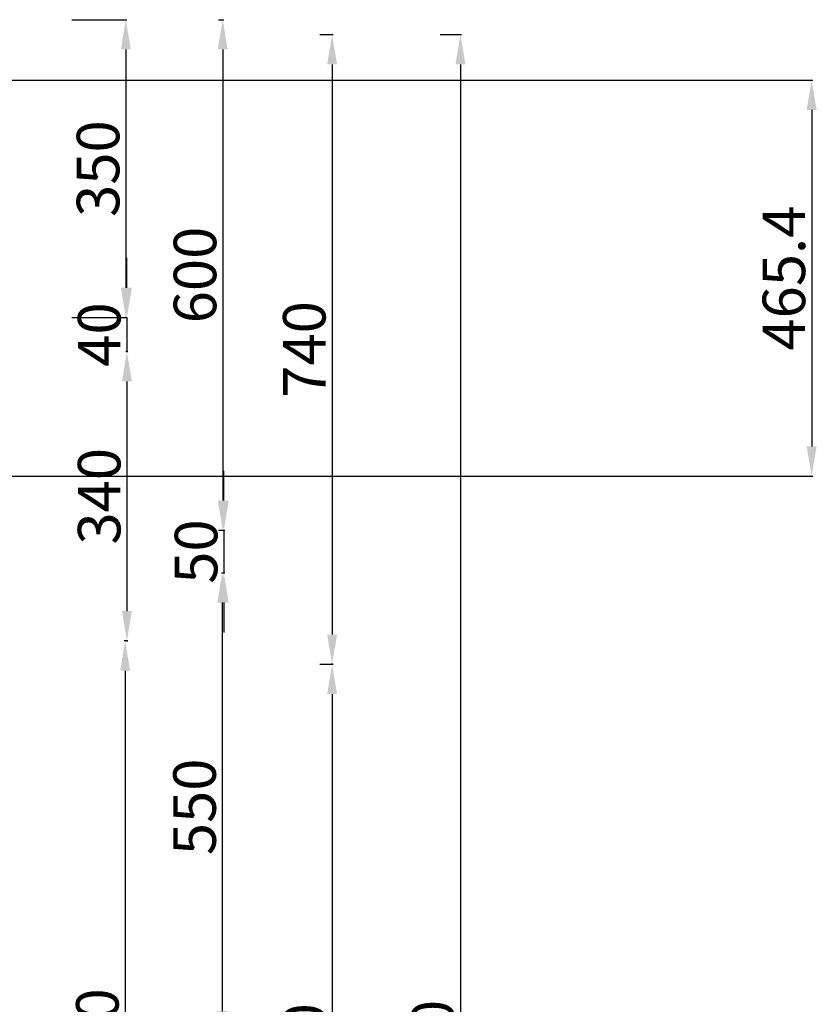
# Model space of a CAD drawing. Units: millimetres. Extents: x 407065 to 421840, y 1168257 to 1177792.
# Tile 10 of 17: x 411029 to 411967, y 1175981 to 1177138. Entities that reach past the tile are written whole.
import ezdxf

# ---------------------------------------------------------------- set-up
doc = ezdxf.new("R2010")
doc.units = ezdxf.units.MM
doc.layers.add('A-ANNO-DIMS', color=6, linetype='Continuous', lineweight=18)
doc.styles.get("Standard").update_dxf_attribs({"font": 'arial.ttf'})
doc.dimstyles.new('ISO-25', dxfattribs={"dimtxt": 50, "dimasz": 35, "dimexe": 1.25, "dimexo": 0.625, "dimtad": 1, "dimdec": 1, "dimtxsty": 'Standard', "dimcen": 35, "dimadec": 0, "dimazin": 0, "dimtfac": 1, "dimtdec": 1, "dimtmove": 0, "dimatfit": 3, "dimfxl": 1, "dimarcsym": 0})

# ---------------------------------------------------------------- blocks, each defined once
blk = doc.blocks.new('*D18')
at = {"layer": 'A-ANNO-DIMS', "color": 0, "lineweight": -2, "transparency": 16777216}
for p, q in [((411090.8, 1177137.8), (411155.4, 1177137.8)), ((411154.2, 1177102.8), (411154.2, 1176822.8)), ((411090.8, 1176787.8), (411155.4, 1176787.8))]:
    blk.add_line(p, q, dxfattribs=at)
at = {"layer": 'A-ANNO-DIMS', "color": 0, "transparency": 16777216}
for points in [[(411148.3, 1177102.8), (411160, 1177102.8), (411154.2, 1177137.8)], [(411148.3, 1176822.8), (411160, 1176822.8), (411154.2, 1176787.8)]]:
    blk.add_solid(points, dxfattribs=at)
at = {"layer": 'Defpoints', "color": 0, "transparency": 16777216}
for p in [(411090.2, 1177137.8), (411090.2, 1176787.8), (411154.2, 1176787.8)]:
    blk.add_point(p, dxfattribs=at)
at = {"layer": 'A-ANNO-DIMS', "color": 0, "transparency": 16777216, "insert": (411128, 1176962.8), "char_height": 50, "attachment_point": 5, "rotation": 90}
blk.add_mtext('350', dxfattribs=at)
blk = doc.blocks.new('*D19')
at = {"layer": 'A-ANNO-DIMS', "color": 0, "lineweight": -2, "transparency": 16777216}
for p, q in [((411155.4, 1176822.8), (411155.4, 1176857.8)), ((411154.8, 1176787.8), (411154.2, 1176787.8)), ((411155.4, 1176787.8), (411155.4, 1176747.8)), ((411154.8, 1176747.8), (411154.2, 1176747.8)), ((411155.4, 1176712.8), (411155.4, 1176677.8))]:
    blk.add_line(p, q, dxfattribs=at)
at = {"layer": 'A-ANNO-DIMS', "color": 0, "transparency": 16777216}
for points in [[(411149.6, 1176822.8), (411161.3, 1176822.8), (411155.4, 1176787.8)], [(411149.6, 1176712.8), (411161.3, 1176712.8), (411155.4, 1176747.8)]]:
    blk.add_solid(points, dxfattribs=at)
at = {"layer": 'Defpoints', "color": 0, "transparency": 16777216}
for p in [(411155.4, 1176787.8), (411155.4, 1176747.8), (411155.4, 1176747.8)]:
    blk.add_point(p, dxfattribs=at)
at = {"layer": 'A-ANNO-DIMS', "color": 0, "transparency": 16777216, "insert": (411129.3, 1176767.8), "char_height": 50, "attachment_point": 5, "rotation": 90}
blk.add_mtext('40', dxfattribs=at)
blk = doc.blocks.new('*D20')
at = {"layer": 'A-ANNO-DIMS', "color": 0, "lineweight": -2, "transparency": 16777216}
for p, q in [((411154.8, 1176747.8), (411156.7, 1176747.8)), ((411155.4, 1176712.8), (411155.4, 1176442.8)), ((411154.8, 1176407.8), (411156.7, 1176407.8))]:
    blk.add_line(p, q, dxfattribs=at)
at = {"layer": 'A-ANNO-DIMS', "color": 0, "transparency": 16777216}
for points in [[(411149.6, 1176712.8), (411161.3, 1176712.8), (411155.4, 1176747.8)], [(411149.6, 1176442.8), (411161.3, 1176442.8), (411155.4, 1176407.8)]]:
    blk.add_solid(points, dxfattribs=at)
at = {"layer": 'Defpoints', "color": 0, "transparency": 16777216}
for p in [(411154.2, 1176747.8), (411154.2, 1176407.8), (411155.4, 1176407.8)]:
    blk.add_point(p, dxfattribs=at)
at = {"layer": 'A-ANNO-DIMS', "color": 0, "transparency": 16777216, "insert": (411129.3, 1176577.8), "char_height": 50, "attachment_point": 5, "rotation": 90}
blk.add_mtext('340', dxfattribs=at)
blk = doc.blocks.new('*D21')
at = {"layer": 'A-ANNO-DIMS', "color": 0, "lineweight": -2, "transparency": 16777216}
for p, q in [((411156.1, 1176407.8), (411152.2, 1176407.8)), ((411153.4, 1176372.8), (411153.4, 1175512.8)), ((411156.1, 1175477.8), (411152.2, 1175477.8))]:
    blk.add_line(p, q, dxfattribs=at)
at = {"layer": 'A-ANNO-DIMS', "color": 0, "transparency": 16777216}
for points in [[(411147.6, 1176372.8), (411159.2, 1176372.8), (411153.4, 1176407.8)], [(411147.6, 1175512.8), (411159.2, 1175512.8), (411153.4, 1175477.8)]]:
    blk.add_solid(points, dxfattribs=at)
at = {"layer": 'Defpoints', "color": 0, "transparency": 16777216}
for p in [(411156.7, 1176407.8), (411153.4, 1175477.8), (411156.7, 1175477.8)]:
    blk.add_point(p, dxfattribs=at)
at = {"layer": 'A-ANNO-DIMS', "color": 0, "transparency": 16777216, "insert": (411127.2, 1175942.8), "char_height": 50, "attachment_point": 5, "rotation": 90}
blk.add_mtext('930', dxfattribs=at)
blk = doc.blocks.new('*D26')
at = {"layer": 'A-ANNO-DIMS', "color": 0, "lineweight": -2, "transparency": 16777216}
for p, q in [((411263.1, 1177137.8), (411269.3, 1177137.8)), ((411268.1, 1177102.8), (411268.1, 1176572.8)), ((411263.1, 1176537.8), (411269.3, 1176537.8))]:
    blk.add_line(p, q, dxfattribs=at)
at = {"layer": 'A-ANNO-DIMS', "color": 0, "transparency": 16777216}
for points in [[(411262.2, 1177102.8), (411273.9, 1177102.8), (411268.1, 1177137.8)], [(411262.2, 1176572.8), (411273.9, 1176572.8), (411268.1, 1176537.8)]]:
    blk.add_solid(points, dxfattribs=at)
at = {"layer": 'Defpoints', "color": 0, "transparency": 16777216}
for p in [(411262.5, 1177137.8), (411262.5, 1176537.8), (411268.1, 1176537.8)]:
    blk.add_point(p, dxfattribs=at)
at = {"layer": 'A-ANNO-DIMS', "color": 0, "transparency": 16777216, "insert": (411241.9, 1176837.8), "char_height": 50, "attachment_point": 5, "rotation": 90}
blk.add_mtext('600', dxfattribs=at)
blk = doc.blocks.new('*D27')
at = {"layer": 'A-ANNO-DIMS', "color": 0, "lineweight": -2, "transparency": 16777216}
for p, q in [((411269.3, 1176572.8), (411269.3, 1176607.8)), ((411266.8, 1176537.8), (411270.6, 1176537.8)), ((411269.3, 1176537.8), (411269.3, 1176487.8)), ((411266.8, 1176487.8), (411270.6, 1176487.8)), ((411269.3, 1176452.8), (411269.3, 1176417.8))]:
    blk.add_line(p, q, dxfattribs=at)
at = {"layer": 'A-ANNO-DIMS', "color": 0, "transparency": 16777216}
for points in [[(411263.5, 1176572.8), (411275.1, 1176572.8), (411269.3, 1176537.8)], [(411263.5, 1176452.8), (411275.1, 1176452.8), (411269.3, 1176487.8)]]:
    blk.add_solid(points, dxfattribs=at)
at = {"layer": 'Defpoints', "color": 0, "transparency": 16777216}
for p in [(411266.2, 1176537.8), (411266.2, 1176487.8), (411269.3, 1176487.8)]:
    blk.add_point(p, dxfattribs=at)
at = {"layer": 'A-ANNO-DIMS', "color": 0, "transparency": 16777216, "insert": (411243.2, 1176512.8), "char_height": 50, "attachment_point": 5, "rotation": 90}
blk.add_mtext('50', dxfattribs=at)
blk = doc.blocks.new('*D28')
at = {"layer": 'A-ANNO-DIMS', "color": 0, "lineweight": -2, "transparency": 16777216}
for p, q in [((411267.4, 1176487.8), (411268.8, 1176487.8)), ((411267.5, 1176452.8), (411267.5, 1175972.8)), ((411267.4, 1175937.8), (411268.8, 1175937.8))]:
    blk.add_line(p, q, dxfattribs=at)
at = {"layer": 'A-ANNO-DIMS', "color": 0, "transparency": 16777216}
for points in [[(411261.7, 1176452.8), (411273.4, 1176452.8), (411267.5, 1176487.8)], [(411261.7, 1175972.8), (411273.4, 1175972.8), (411267.5, 1175937.8)]]:
    blk.add_solid(points, dxfattribs=at)
at = {"layer": 'Defpoints', "color": 0, "transparency": 16777216}
for p in [(411266.8, 1176487.8), (411266.8, 1175937.8), (411267.5, 1175937.8)]:
    blk.add_point(p, dxfattribs=at)
at = {"layer": 'A-ANNO-DIMS', "color": 0, "transparency": 16777216, "insert": (411241.4, 1176212.8), "char_height": 50, "attachment_point": 5, "rotation": 90}
blk.add_mtext('550', dxfattribs=at)
blk = doc.blocks.new('*D31')
at = {"layer": 'A-ANNO-DIMS', "color": 0, "lineweight": -2, "transparency": 16777216}
for p, q in [((411382.2, 1177120.3), (411397.8, 1177120.3)), ((411396.6, 1177085.3), (411396.6, 1176415.3)), ((411382.2, 1176380.3), (411397.8, 1176380.3))]:
    blk.add_line(p, q, dxfattribs=at)
at = {"layer": 'A-ANNO-DIMS', "color": 0, "transparency": 16777216}
for points in [[(411390.8, 1177085.3), (411402.4, 1177085.3), (411396.6, 1177120.3)], [(411390.8, 1176415.3), (411402.4, 1176415.3), (411396.6, 1176380.3)]]:
    blk.add_solid(points, dxfattribs=at)
at = {"layer": 'Defpoints', "color": 0, "transparency": 16777216}
for p in [(411381.6, 1177120.3), (411381.6, 1176380.3), (411396.6, 1176380.3)]:
    blk.add_point(p, dxfattribs=at)
at = {"layer": 'A-ANNO-DIMS', "color": 0, "transparency": 16777216, "insert": (411370.4, 1176750.3), "char_height": 50, "attachment_point": 5, "rotation": 90}
blk.add_mtext('740', dxfattribs=at)
blk = doc.blocks.new('*D32')
at = {"layer": 'A-ANNO-DIMS', "color": 0, "lineweight": -2, "transparency": 16777216}
for p, q in [((411397.2, 1176380.3), (411395.3, 1176380.3)), ((411396.6, 1176345.3), (411396.6, 1175505.3)), ((411397.2, 1175470.3), (411395.3, 1175470.3))]:
    blk.add_line(p, q, dxfattribs=at)
at = {"layer": 'A-ANNO-DIMS', "color": 0, "transparency": 16777216}
for points in [[(411390.8, 1176345.3), (411402.4, 1176345.3), (411396.6, 1176380.3)], [(411390.8, 1175505.3), (411402.4, 1175505.3), (411396.6, 1175470.3)]]:
    blk.add_solid(points, dxfattribs=at)
at = {"layer": 'Defpoints', "color": 0, "transparency": 16777216}
for p in [(411397.8, 1176380.3), (411396.6, 1175470.3), (411397.8, 1175470.3)]:
    blk.add_point(p, dxfattribs=at)
at = {"layer": 'A-ANNO-DIMS', "color": 0, "transparency": 16777216, "insert": (411370.4, 1175925.3), "char_height": 50, "attachment_point": 5, "rotation": 90}
blk.add_mtext('910', dxfattribs=at)
blk = doc.blocks.new('*D34')
at = {"layer": 'A-ANNO-DIMS', "color": 0, "lineweight": -2, "transparency": 16777216}
for p, q in [((411523.7, 1177120.3), (411548.7, 1177120.3)), ((411547.4, 1177085.3), (411547.4, 1174735.3)), ((411523.7, 1174700.3), (411548.7, 1174700.3))]:
    blk.add_line(p, q, dxfattribs=at)
at = {"layer": 'A-ANNO-DIMS', "color": 0, "transparency": 16777216}
for points in [[(411541.6, 1177085.3), (411553.3, 1177085.3), (411547.4, 1177120.3)], [(411541.6, 1174735.3), (411553.3, 1174735.3), (411547.4, 1174700.3)]]:
    blk.add_solid(points, dxfattribs=at)
at = {"layer": 'Defpoints', "color": 0, "transparency": 16777216}
for p in [(411523.1, 1177120.3), (411523.1, 1174700.3), (411547.4, 1174700.3)]:
    blk.add_point(p, dxfattribs=at)
at = {"layer": 'A-ANNO-DIMS', "color": 0, "transparency": 16777216, "insert": (411521.3, 1175910.3), "char_height": 50, "attachment_point": 5, "rotation": 90}
blk.add_mtext('2420', dxfattribs=at)
blk = doc.blocks.new('*D179')
at = {"layer": 'A-ANNO-DIMS', "color": 0, "lineweight": -2, "transparency": 16777216}
for p, q in [((409943.6, 1177066.8), (411961.4, 1177066.8)), ((411960.2, 1177031.8), (411960.2, 1176636.4)), ((409943.6, 1176601.4), (411961.4, 1176601.4))]:
    blk.add_line(p, q, dxfattribs=at)
at = {"layer": 'A-ANNO-DIMS', "color": 0, "transparency": 16777216}
for points in [[(411954.3, 1177031.8), (411966, 1177031.8), (411960.2, 1177066.8)], [(411954.3, 1176636.4), (411966, 1176636.4), (411960.2, 1176601.4)]]:
    blk.add_solid(points, dxfattribs=at)
at = {"layer": 'Defpoints', "color": 0, "transparency": 16777216}
for p in [(409943, 1177066.8), (409943, 1176601.4), (411960.2, 1176601.4)]:
    blk.add_point(p, dxfattribs=at)
at = {"layer": 'A-ANNO-DIMS', "color": 0, "transparency": 16777216, "insert": (411934, 1176834.1), "char_height": 50, "attachment_point": 5, "rotation": 90}
blk.add_mtext('465.4', dxfattribs=at)

msp = doc.modelspace()

# ---------------------------------------------------------------- dimensions: what is measured, and where the dimension line sits
at = {"layer": 'A-ANNO-DIMS'}
for base, p1, p2, override, picture, middle in [((411154.1757, 1176787.7952), (411090.182, 1177137.7952), (411090.182, 1176787.7952), {"dimclrd": 0, "dimclre": 0, "dimclrt": 0}, '*D18', (411128.005, 1176962.7952)), ((411268.0598, 1176537.7952), (411262.4536, 1177137.7952), (411262.4536, 1176537.7952), {"dimclrd": 0, "dimclre": 0, "dimclrt": 0}, '*D26', (411241.9061, 1176837.7952)), ((411396.5925, 1176380.2952), (411381.5589, 1177120.2952), (411381.5589, 1176380.2952), {"dimclrd": 0, "dimclre": 0, "dimclrt": 0}, '*D31', (411370.4388, 1176750.2952)), ((411547.4266, 1174700.2952), (411523.1043, 1177120.2952), (411523.1043, 1174700.2952), {"dimclrd": 0, "dimclre": 0, "dimclrt": 0}, '*D34', (411521.2729, 1175910.2952)), ((411960.1736, 1176601.4062), (409942.9713, 1177066.8168), (409942.9713, 1176601.4062), {"dimdec": 1, "dimlfac": 1, "dimrnd": 0, "dimzin": 0, "dimdsep": 46, "dimlunit": 2}, '*D179', (411934.02, 1176834.1115)), ((411155.4257, 1176407.7952), (411154.1757, 1176747.7952), (411154.1757, 1176407.7952), {"dimclrd": 0, "dimclre": 0, "dimclrt": 0}, '*D20', (411129.255, 1176577.7952)), ((411267.522, 1175937.7952), (411266.8192, 1176487.7952), (411266.8192, 1175937.7952), {"dimclrd": 0, "dimclre": 0, "dimclrt": 0}, '*D28', (411241.3684, 1176212.7952)), ((411153.4065, 1175477.7952), (411156.6757, 1176407.7952), (411156.6757, 1175477.7952), {"dimclrd": 0, "dimclre": 0, "dimclrt": 0}, '*D21', (411127.2358, 1175942.7952)), ((411396.5925, 1175470.2952), (411397.8425, 1176380.2952), (411397.8425, 1175470.2952), {"dimclrd": 0, "dimclre": 0, "dimclrt": 0}, '*D32', (411370.4388, 1175925.2952))]:
    dim = msp.add_linear_dim(base=base, p1=p1, p2=p2, angle=90, dimstyle='ISO-25', override=override, dxfattribs=at)
    dim.commit()
    dim.dimension.update_dxf_attribs({"geometry": picture, "text_midpoint": middle})
for base, p1, p2, picture, middle in [((411155.4257, 1176747.7952), (411155.4257, 1176787.7952), (411155.4257, 1176747.7952), '*D19', (411155.4257, 1176767.7952)), ((411269.3098, 1176487.7952), (411266.1942, 1176537.7952), (411266.1942, 1176487.7952), '*D27', (411269.3098, 1176512.7952))]:
    dim = msp.add_linear_dim(base=base, p1=p1, p2=p2, angle=90, dimstyle='ISO-25', override={"dimclrd": 0, "dimclre": 0, "dimclrt": 0}, dxfattribs=at)
    dim.commit()
    dim.dimension.update_dxf_attribs({"geometry": picture, "text_midpoint": middle, "dimtype": 160})

doc.saveas('drawing.dxf')
